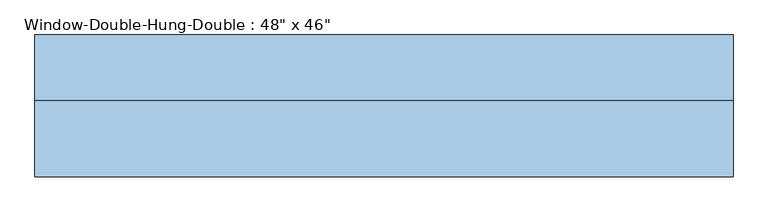
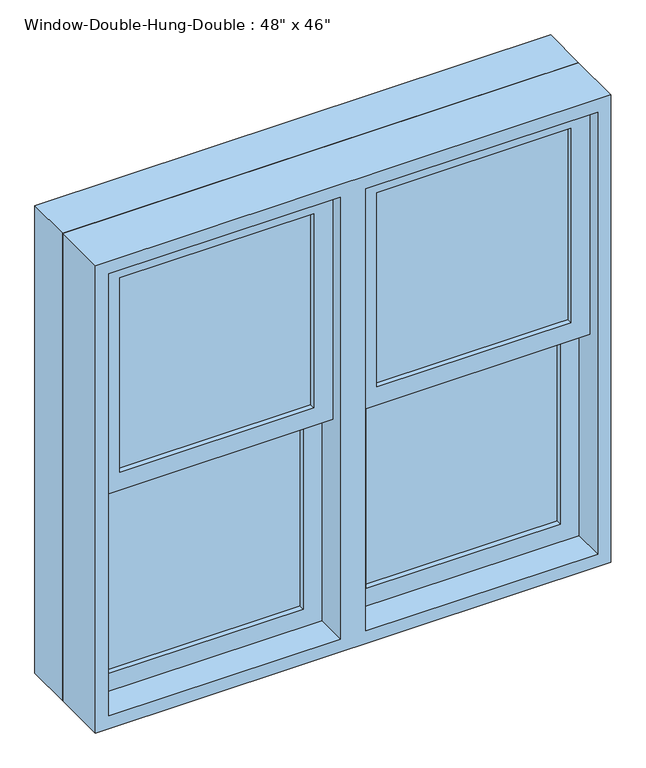
"""IFC4 building model written with IfcOpenShell, lengths in millimetres: window geometry."""

from ifc_helpers import new_model, si_unit, frame, origin, place, context, project, spatial, polyline, outline, extrude, source, transform, mapped, element, save


def window_25281ba2(model_context):
    return source(origin(), model_context, "Body", "SweptSolid", [
        extrude(outline(polyline([(2082.8, 609.6), (2082.8, -609.6), (914.4, -609.6), (914.4, 609.6), (2082.8, 609.6)]), holes=[polyline([(2063.75, 590.55), (933.45, 590.55), (933.45, -590.55), (2063.75, -590.55), (2063.75, 590.55)])]), frame((0.0, 0.0, 0.0), z_axis=(0.0, 1.0, 0.0), x_axis=(0.0, 0.0, 1.0)), (0.0, 0.0, 1.0), 114.3),
        extrude(outline(polyline([(2051.05, 577.85), (2051.05, 30.1625), (1476.375, 30.1625), (1476.375, 577.85), (2051.05, 577.85)]), holes=[polyline([(2006.6, 74.6125), (2006.6, 533.4), (1520.825, 533.4), (1520.825, 74.6125), (2006.6, 74.6125)])]), frame((0.0, -101.6, 0.0), z_axis=(0.0, 1.0, 0.0), x_axis=(0.0, 0.0, 1.0)), (0.0, 0.0, 1.0), 44.45),
        extrude(outline(polyline([(1520.825, 577.85), (1520.825, 30.1625), (946.15, 30.1625), (946.15, 577.85), (1520.825, 577.85)]), holes=[polyline([(1476.375, 74.6125), (1476.375, 533.4), (990.6, 533.4), (990.6, 74.6125), (1476.375, 74.6125)])]), frame((0.0, -57.15, 0.0), z_axis=(0.0, 1.0, 0.0), x_axis=(0.0, 0.0, 1.0)), (0.0, 0.0, 1.0), 44.45),
        extrude(outline(polyline([(533.4, -88.9), (74.6125, -88.9), (74.6125, -82.55), (533.4, -82.55), (533.4, -88.9)])), frame((0.0, 0.0, 1520.825), z_axis=(0.0, 0.0, 1.0), x_axis=(1.0, 0.0, 0.0)), (0.0, 0.0, 1.0), 485.775),
        extrude(outline(polyline([(74.6125, -76.2), (74.6125, -69.85), (533.4, -69.85), (533.4, -76.2), (74.6125, -76.2)])), frame((0.0, 0.0, 1520.825), z_axis=(0.0, 0.0, 1.0), x_axis=(1.0, 0.0, 0.0)), (0.0, 0.0, 1.0), 485.775),
        extrude(outline(polyline([(533.4, -44.45), (74.6125, -44.45), (74.6125, -38.1), (533.4, -38.1), (533.4, -44.45)])), frame((0.0, 0.0, 990.6), z_axis=(0.0, 0.0, 1.0), x_axis=(1.0, 0.0, 0.0)), (0.0, 0.0, 1.0), 485.775),
        extrude(outline(polyline([(74.6125, -31.75), (74.6125, -25.4), (533.4, -25.4), (533.4, -31.75), (74.6125, -31.75)])), frame((0.0, 0.0, 990.6), z_axis=(0.0, 0.0, 1.0), x_axis=(1.0, 0.0, 0.0)), (0.0, 0.0, 1.0), 485.775),
        extrude(outline(polyline([(2051.05, -30.1625), (2051.05, -577.85), (1476.375, -577.85), (1476.375, -30.1625), (2051.05, -30.1625)]), holes=[polyline([(2006.6, -533.4), (2006.6, -74.6125), (1520.825, -74.6125), (1520.825, -533.4), (2006.6, -533.4)])]), frame((0.0, -101.6, 0.0), z_axis=(0.0, 1.0, 0.0), x_axis=(0.0, 0.0, 1.0)), (0.0, 0.0, 1.0), 44.45),
        extrude(outline(polyline([(1520.825, -30.1625), (1520.825, -577.85), (946.15, -577.85), (946.15, -30.1625), (1520.825, -30.1625)]), holes=[polyline([(1476.375, -533.4), (1476.375, -74.6125), (990.6, -74.6125), (990.6, -533.4), (1476.375, -533.4)])]), frame((0.0, -57.15, 0.0), z_axis=(0.0, 1.0, 0.0), x_axis=(0.0, 0.0, 1.0)), (0.0, 0.0, 1.0), 44.45),
        extrude(outline(polyline([(-533.4, -88.9), (-533.4, -82.55), (-74.6125, -82.55), (-74.6125, -88.9), (-533.4, -88.9)])), frame((0.0, 0.0, 1520.825), z_axis=(0.0, 0.0, 1.0), x_axis=(1.0, 0.0, 0.0)), (0.0, 0.0, 1.0), 485.775),
        extrude(outline(polyline([(-74.6125, -76.2), (-533.4, -76.2), (-533.4, -69.85), (-74.6125, -69.85), (-74.6125, -76.2)])), frame((0.0, 0.0, 1520.825), z_axis=(0.0, 0.0, 1.0), x_axis=(1.0, 0.0, 0.0)), (0.0, 0.0, 1.0), 485.775),
        extrude(outline(polyline([(-533.4, -44.45), (-533.4, -38.1), (-74.6125, -38.1), (-74.6125, -44.45), (-533.4, -44.45)])), frame((0.0, 0.0, 990.6), z_axis=(0.0, 0.0, 1.0), x_axis=(1.0, 0.0, 0.0)), (0.0, 0.0, 1.0), 485.775),
        extrude(outline(polyline([(-74.6125, -31.75), (-533.4, -31.75), (-533.4, -25.4), (-74.6125, -25.4), (-74.6125, -31.75)])), frame((0.0, 0.0, 990.6), z_axis=(0.0, 0.0, 1.0), x_axis=(1.0, 0.0, 0.0)), (0.0, 0.0, 1.0), 485.775),
        extrude(outline(polyline([(2082.8, -609.6), (914.4, -609.6), (914.4, 609.6), (2082.8, 609.6), (2082.8, -609.6)]), holes=[polyline([(2051.05, -577.85), (2051.05, -30.1625), (946.15, -30.1625), (946.15, -577.85), (2051.05, -577.85)]), polyline([(2051.05, 577.85), (946.15, 577.85), (946.15, 30.1625), (2051.05, 30.1625), (2051.05, 577.85)])]), frame((0.0, -133.35, 0.0), z_axis=(0.0, 1.0, 0.0), x_axis=(0.0, 0.0, 1.0)), (0.0, 0.0, 1.0), 133.35),
    ])


if __name__ == "__main__":
    model = new_model("IFC4")
    model_context = context("Model", 3, world=origin())
    ifc_project = project(units=[si_unit("LENGTHUNIT", "METRE", prefix="MILLI")], contexts=[model_context])
    site = spatial("IfcSite", under=ifc_project)
    building = spatial("IfcBuilding", under=site)
    placement = place(None, origin())
    window_shape = window_25281ba2(model_context)
    element("IfcWindow", 1, ObjectType="Window-Double-Hung-Double : 48\" x 46\"", at=placement, inside=building, context=model_context, shape_type="MappedRepresentation", body=[
        mapped(window_shape, transform((0.0, 0.0, 0.0), x_axis=(1.0, 0.0, 0.0), y_axis=(0.0, 1.0, 0.0), z_axis=(0.0, 0.0, 1.0))),
    ])
    save(model, "model.ifc")

# Revit data of these elements
# Type "Window-Double-Hung-Double : 48\" x 46\""
#   Type Mark = "21"
#   Fire Rating = "0.5h"
#   Construction Type Id = "DG-DR"
#   Assembly Code = "B2020100"
#   Analytic Construction = "Double glazing - domestic"
#   Wall Thickness [instance default] = 0' - 6"
#   Window Inset [instance default] = 0' - 0"
#   Visual Light Transmittance = 0.81
#   Thermal Resistance (R) = 1.8146 (h·ft²·°F)/BTU
#   Solar Heat Gain Coefficient = 0.76
#   Muntin Width = 1' - 6 1/16"
#   Muntin Height = 1' - 7 1/8"
#   Interior Wall Closure [instance default] = 0' - 1 1/2"
#   Rough Width = 4' - 0 1/2"
#   Rough Height = 3' - 10 1/2"
#   Frame Extension [instance default] = 0' - 1 1/4"
#   Exterior Wall Closure [instance default] = 0' - 0 1/2"
#   Extension Jamb [instance default] = 0' - 1 1/2"
#   Heat Transfer Coefficient (U) = 0.5511 BTU/(h·ft²·°F)
#   Height = 3' - 10"
#   Width = 4' - 0"
#   Top Muntin Visibility = yes
#   Indicator Visibility [instance default] = yes
#   Extension Jamb Visibility [instance default] = yes
#   Interior Trim Visibility [instance default] = yes
#   Exterior Trim Visibility [instance default] = yes
#   Define Thermal Properties by = 1
#   Bottom Muntin Visibility = yes
#   Muntin Pattern = Muntin Pattern_2x2 : Muntin Pattern_2x2
#   Interior Trim Material = Wood - Stained
#   Interior Trim = Trim-Window-Interior-Flat : Picture Frame
#   Exterior Trim Material = Clad - White
#   Exterior Trim = Trim-Window-Exterior-Flat : with Sill
#   Glass Panel Material = Glass
#   Exterior Frame Material = Clad - White
#   Interior Frame Material = Wood - Stained
#   Wall Closure = (empty or 0)
# Element 1 (IfcWindow, "Window-Double-Hung-Double : 48\" x 46\"")
#   Wall Thickness = 0' - 9"
#   Extension Jamb = 0' - 4 1/2"
#   Materials on its faces: "Wood - Stained", "Glass", "Clad - White"
# Materials
#   "Wood - Stained": class "Wood", colour RGB 224 178 126, transparency 0, Cost = 0
#   "Clad - White": class "Wood", colour RGB 242 242 238, transparency 0, Cost = 0
#   "Glass": class "Glass", colour RGB 0 128 192, transparency 0.75, Description = "Soda Lime Glass", Cost = 0
